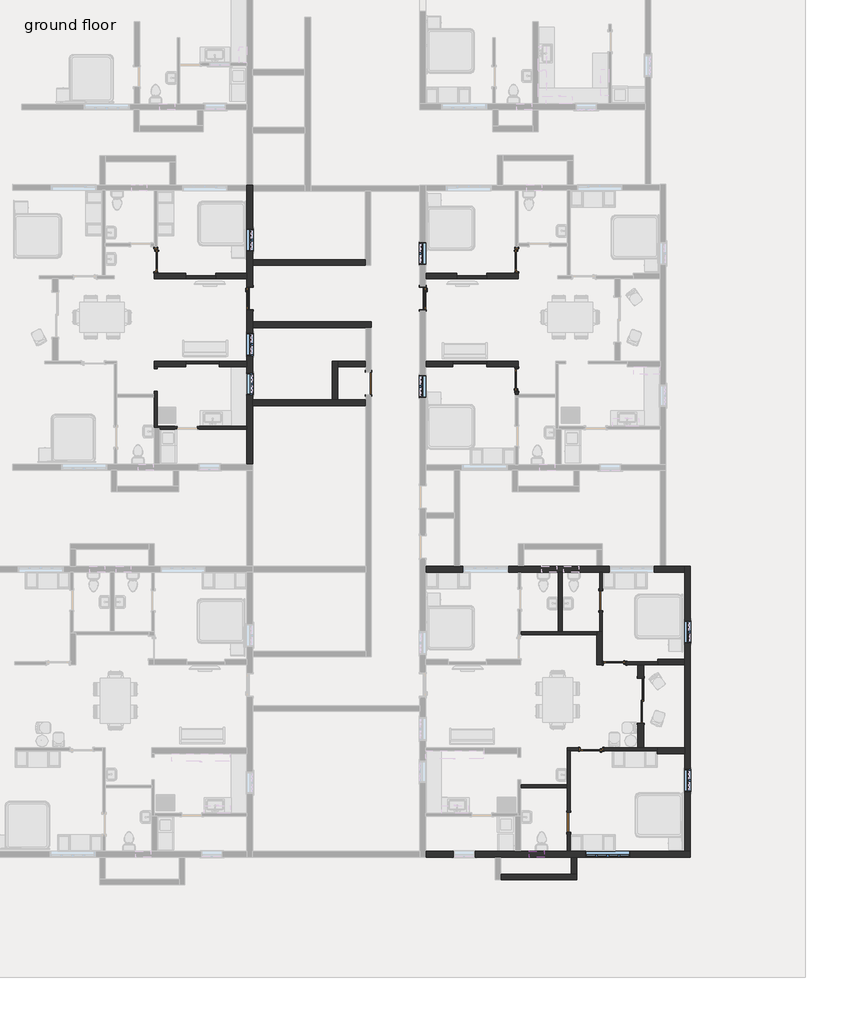
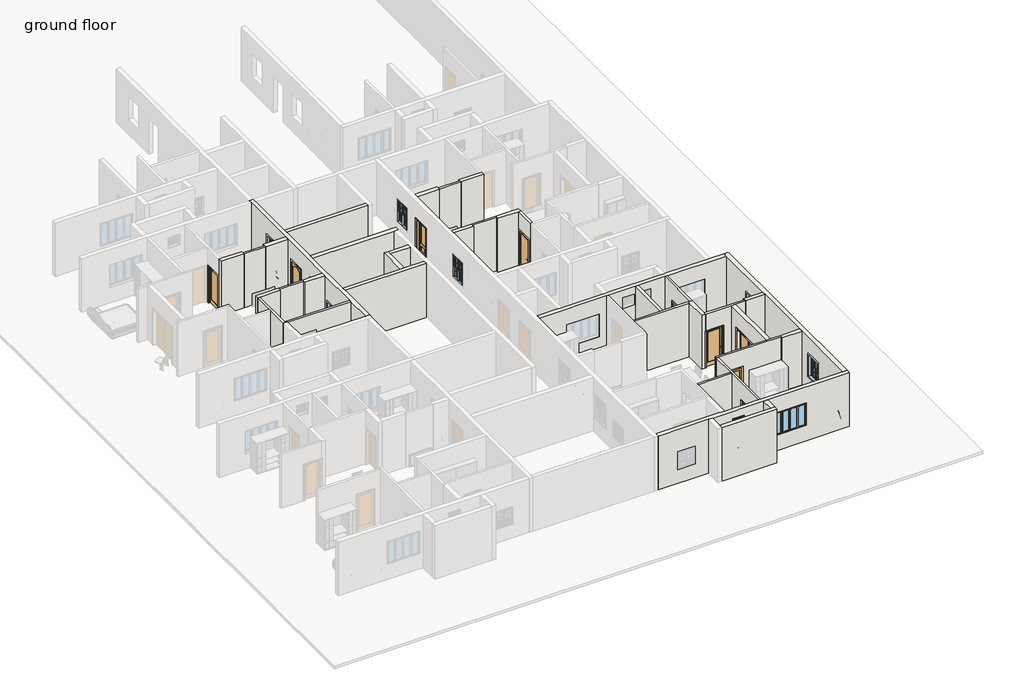
# One storey, part 3 of 16: 37 walls, 11 doors, 9 windows.
# Revit data of these elements (continued)
# Type "Window-Single-Hung-Double : 36\" x 52\"" (continued)
#   Construction Type Id = "DG-DR"
#   Assembly Code = "B2020100"
#   Analytic Construction = "Double glazing - domestic"
#   Wall Thickness [instance default] = 0' - 6"
#   Window Inset [instance default] = 0' - 0"
#   Visual Light Transmittance = 0.81
#   Thermal Resistance (R) = 1.8146 (h·ft²·°F)/BTU
#   Solar Heat Gain Coefficient = 0.76
#   Muntin Width = 1' - 0 1/16"
#   Muntin Height = 1' - 10 1/8"
#   Interior Wall Closure [instance default] = 0' - 1 1/2"
#   Rough Width = 3' - 0 1/2"
#   Rough Height = 4' - 4 1/2"
#   Frame Extension [instance default] = 0' - 1 1/4"
#   Exterior Wall Closure [instance default] = 0' - 0 1/2"
#   Extension Jamb [instance default] = 0' - 1 1/2"
#   Heat Transfer Coefficient (U) = 0.5511 BTU/(h·ft²·°F)
#   Height = 4' - 4"
#   Width = 3' - 0"
#   Top Muntin Visibility = yes
#   Indicator Visibility [instance default] = yes
#   Extension Jamb Visibility [instance default] = yes
#   Interior Trim Visibility [instance default] = yes
#   Exterior Trim Visibility [instance default] = yes
#   Define Thermal Properties by = 1
#   Bottom Muntin Visibility = yes
#   Muntin Pattern = Muntin Pattern_2x2 : Muntin Pattern_2x2
#   Interior Trim = Trim-Window-Interior-Flat : Picture Frame
#   Interior Trim Material = Wood - Stained
#   Exterior Trim Material = Clad - White
#   Exterior Trim = Trim-Window-Exterior-Flat : with Sill
#   Glass Panel Material = Glass
#   Exterior Frame Material = Clad - White
#   Interior Frame Material = Wood - Stained
#   Wall Closure = (empty or 0)
# Elements 1, 2 (IfcDoor, "36\" x 84\"")
#   Threshold Offset = 0' - 0 1/2"
#   Swing Angle = 90.00°
#   Door Offset = 0' - 0"
#   Threshold = yes
#   Exterior Trim = yes
#   Phase Created = New Construction
#   Materials on its faces: "Cherry", "Aluminum", "Glass"
# Element 3 (IfcDoor, "Door-Double-Sliding : 72\" x 84\"")
#   Phase Created = New Construction
#   Materials on its faces: "Paint - Sienna", "Wood - Birch - Solid Stained Light Low Gloss", "Glass"
# Elements 4, 5, 6, 7, 8 (IfcDoor, "Door-Interior-Single-1_Panel-Wood : 36\" x 84\"")
#   Swing Angle = 90.00°
#   Phase Created = New Construction
#   Materials on its faces: "Cherry", "Aluminum"
# Elements 9, 10 (IfcDoor, "Single-Flush : 32\" x 84\"")
#   Phase Created = New Construction
#   Materials on its faces: "Door - Frame", "Door - Panel"
# Element 11 (IfcDoor, "Single-Flush : 36\" x 84\"")
#   Phase Created = New Construction
#   Materials on its faces: "Door - Frame", "Door - Panel"
# Elements 12, 13, 14, 15, 16, 17, 18, 19, 20, 21, 22, 23, 24 (IfcWall, "Generic - 4.5\"")
#   Top Offset = 0' - 0"
#   Base Offset = 0' - 0"
#   wall height = 10' - 6"
#   Phase Created = New Construction
#   Base Constraint = ground floor
#   Top Constraint = 1st floor
#   Materials on its faces: "Default Wall"
# Element 25 (IfcWall, "Generic - 6\"")
#   Top Offset = 0' - 0"
#   Base Offset = 0' - 0"
#   wall height = 10' - 6"
#   Phase Created = New Construction
#   Base Constraint = ground floor
#   Top Constraint = 1st floor
#   Materials on its faces: "Default Wall"
# Elements 26, 27, 28, 29, 30, 31, 32, 33, 34, 35, 36, 37, 38, 39, 40, 41, 42, 43, 44, 45, 46, 47, 48 (IfcWall, "Generic - 9\"")
#   Top Offset = 0' - 0"
#   Base Offset = 0' - 0"
#   wall height = 10' - 6"
#   Phase Created = New Construction
#   Base Constraint = ground floor
#   Top Constraint = 1st floor
#   Materials on its faces: "Default Wall"
# Element 49 (IfcWindow, "Window-Casement-Double-Awning : 34\" x 36\"")
#   Mark = "84"
#   Window Inset = 0' - 0"
#   Interior Wall Closure = 0' - 2 1/4"
#   Frame Extension = 0' - 0 1/4"
#   Exterior Wall Closure = 0' - 1 1/4"
#   Interior Trim Visibility = yes
#   Exterior Trim Visibility = yes
#   Phase Created = New Construction
#   Materials on its faces: "Wood - Stained", "Glass", "Clad - White"
# Element 50 (IfcWindow, "Window-Casement-Multi-Sash-Horizontal : 72\" x 53\"")
#   Mark = "69"
#   Window Inset = 0' - 0 5/8"
#   Frame Gap 3 = 0' - 1 83/128"
#   Frame Gap 2 = 0' - 0 5/8"
#   Phase Created = New Construction
#   Materials on its faces: "Metal - Aluminum", "Glass"
# Element 51 (IfcWindow, "Window-Louvers : 24\" x 24\"")
#   Mark = "102"
#   Blade Width = 1' - 10 1/2"
#   Phase Created = New Construction
#   Materials on its faces: "Birch"
# Element 52 (IfcWindow, "Window-Single-Hung-Double : 36\" x 52\"")
#   Mark = "51"
#   Window Inset = 0' - 0"
#   Interior Wall Closure = 0' - 1 1/2"
#   Frame Extension = 0' - 1 1/4"
#   Exterior Wall Closure = 0' - 0 1/2"
#   Interior Trim Visibility = yes
#   Indicator Visibility = yes
#   Exterior Trim Visibility = yes
#   Phase Created = New Construction
#   Materials on its faces: "Wood - Stained", "Glass", "Clad - White"
# Element 53 (IfcWindow, "Window-Single-Hung-Double : 36\" x 52\"")
#   Mark = "52"
#   Window Inset = 0' - 0"
#   Interior Wall Closure = 0' - 1 1/2"
#   Frame Extension = 0' - 1 1/4"
#   Exterior Wall Closure = 0' - 0 1/2"
#   Interior Trim Visibility = yes
#   Indicator Visibility = yes
#   Exterior Trim Visibility = yes
#   Phase Created = New Construction
#   Materials on its faces: "Wood - Stained", "Glass", "Clad - White"
# Element 54 (IfcWindow, "Window-Single-Hung-Double : 36\" x 52\"")
#   Mark = "53"
#   Window Inset = 0' - 0"
#   Interior Wall Closure = 0' - 1 1/2"
#   Frame Extension = 0' - 1 1/4"
#   Exterior Wall Closure = 0' - 0 1/2"
#   Interior Trim Visibility = yes
#   Indicator Visibility = yes
#   Exterior Trim Visibility = yes
#   Phase Created = New Construction
#   Materials on its faces: "Wood - Stained", "Glass", "Clad - White"
# Element 55 (IfcWindow, "Window-Single-Hung-Double : 36\" x 52\"")
#   Mark = "60"
#   Window Inset = 0' - 0"
#   Interior Wall Closure = 0' - 1 1/2"
#   Frame Extension = 0' - 1 1/4"
#   Exterior Wall Closure = 0' - 0 1/2"
#   Interior Trim Visibility = yes
#   Indicator Visibility = yes
#   Exterior Trim Visibility = yes
#   Phase Created = New Construction
#   Materials on its faces: "Wood - Stained", "Glass", "Clad - White"
# Element 56 (IfcWindow, "Window-Single-Hung-Double : 36\" x 52\"")
#   Mark = "85"
#   Window Inset = 0' - 0"
#   Interior Wall Closure = 0' - 1 1/2"
#   Frame Extension = 0' - 1 1/4"
#   Exterior Wall Closure = 0' - 0 1/2"
#   Interior Trim Visibility = yes
#   Indicator Visibility = yes
#   Exterior Trim Visibility = yes
#   Phase Created = New Construction
#   Materials on its faces: "Wood - Stained", "Glass", "Clad - White"
# Element 57 (IfcWindow, "Window-Single-Hung-Double : 36\" x 52\"")
#   Mark = "86"
#   Window Inset = 0' - 0"
#   Interior Wall Closure = 0' - 1 1/2"
#   Frame Extension = 0' - 1 1/4"
#   Exterior Wall Closure = 0' - 0 1/2"
#   Interior Trim Visibility = yes
#   Indicator Visibility = yes
#   Exterior Trim Visibility = yes
#   Phase Created = New Construction
#   Materials on its faces: "Wood - Stained", "Glass", "Clad - White"
# Materials
#   "Cherry": class "Wood", colour RGB 226 177 128, transparency 0, Description = "Prunus Serotina", Cost = 0
#   "Glass": class "Glass", colour RGB 0 128 192, transparency 0.75, Description = "Soda Lime Glass", Cost = 0
#   "Aluminum": class "Metal", colour RGB 247 247 247, transparency 0, Description = "Aluminum 6061", Cost = 0
#   "Wood - Birch - Solid Stained Light Low Gloss": class "Wood", colour RGB 210 159 95, transparency 0, Cost = 0
#   "Paint - Sienna": colour RGB 118 70 51, transparency 0, Cost = 0
#   "Door - Panel": class "Wood", colour RGB 210 159 95, transparency 0, Cost = 0
#   "Door - Frame": colour RGB 118 70 51, transparency 0, Cost = 0
#   "Wood - Stained": class "Wood", colour RGB 224 178 126, transparency 0, Cost = 0
#   "Clad - White": class "Wood", colour RGB 242 242 238, transparency 0, Cost = 0
#   "Metal - Aluminum": class "Metal", colour RGB 247 247 247, transparency 0
#   "Birch": class "Wood", colour RGB 224 178 126, transparency 0, Description = "Betula Alleghaniensis", Cost = 0
#   "Default Wall": colour RGB 128 128 128, transparency 0, Cost = 0
